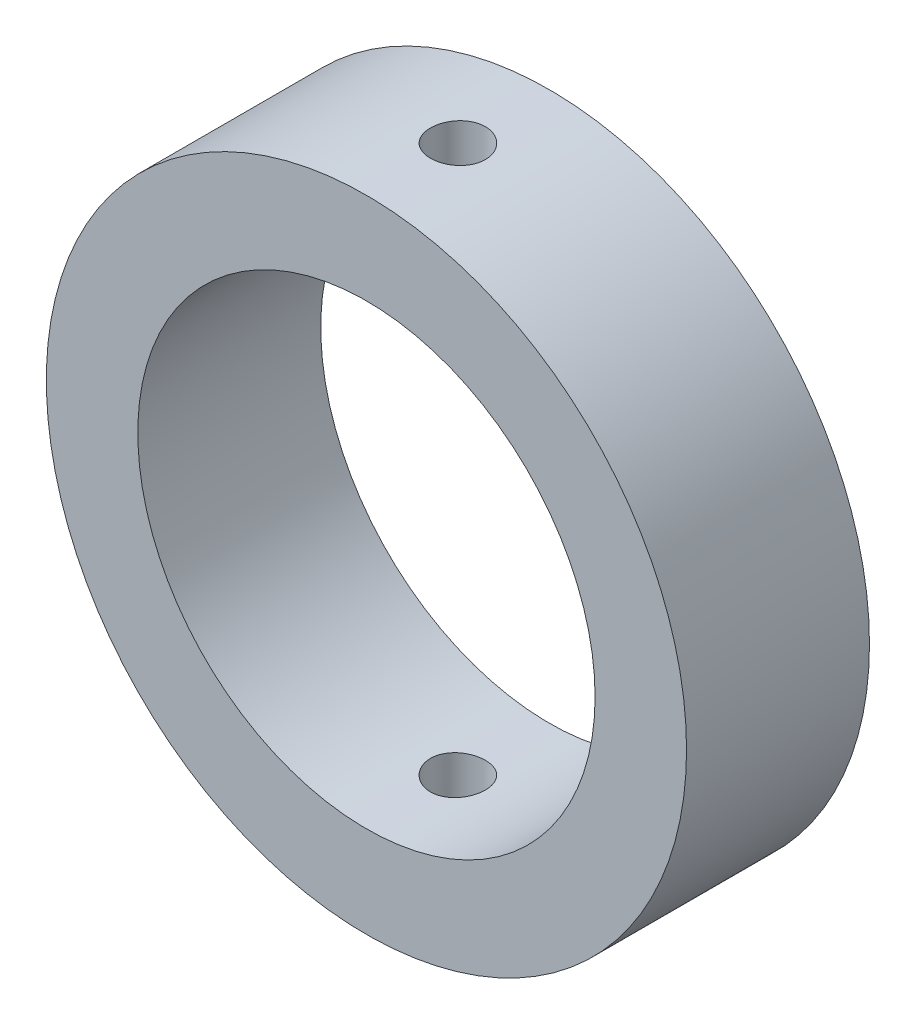
SolidWorks part; units mm, degrees
material "Plain Carbon Steel"
ref_plane "Front Plane" through (0, 0, 0) normal (0, 0, 1) x (1, 0, 0)
ref_plane "Top Plane" through (0, 0, 0) normal (0, 1, 0) x (1, 0, 0)
ref_plane "Right Plane" through (0, 0, 0) normal (1, 0, 0) x (0, 0, -1)
sketch "Collar Ring Sketch Ø70-Ø50" plane through (0, 0, 0) normal (0, 0, 1) x (1, 0, 0)
  circle A0 centre (0, 0) radius 35
  circle A1 centre (0, 0) radius 25
  dimension "D1" = 70
  dimension "D2" = 50
extrude "Collar Ring 20 Thick" add sketch "Collar Ring Sketch Ø70-Ø50" along normal blind 20
sketch "Pin Hole Sketch Ø6" plane through (0, 0, 0) normal (0, 1, 0) x (1, 0, 0)
  line L0 (35, 0) -> (-35, 0) construction
  circle A0 centre (0, -10) radius 3
  dimension "D1" = 6
  dimension "D2" = 10
extrude "Radial Pin Hole Ø6" cut sketch "Pin Hole Sketch Ø6" against normal through all both and the other way through all
